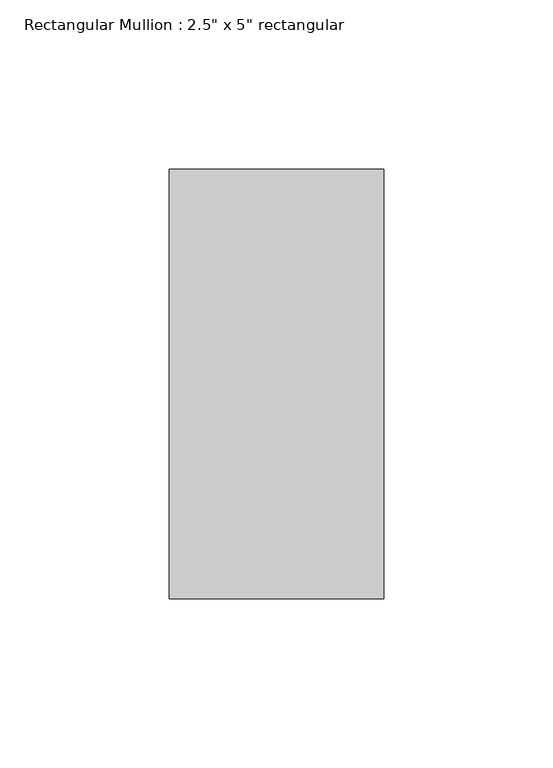
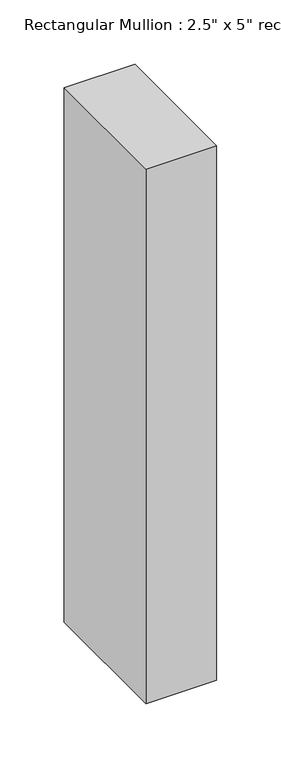
"""IFC4 building model written with IfcOpenShell, lengths in millimetres: member geometry."""

from ifc_helpers import new_model, si_unit, frame, origin, place, context, project, spatial, polyline, outline, extrude, source, transform, mapped, element, save


def member_de31af64(model_context):
    return source(origin(), model_context, "Body", "SweptSolid", [
        extrude(outline(polyline([(0.0, 63.5), (0.0, -63.5), (-63.5, -63.5), (-63.5, 63.5), (0.0, 63.5)])), frame((0.0, 0.0, -506.9149218), z_axis=(0.0, 0.0, 1.0), x_axis=(1.0, 0.0, 0.0)), (0.0, 0.0, 1.0), 506.9149218),
    ])


if __name__ == "__main__":
    model = new_model("IFC4")
    model_context = context("Model", 3, world=origin())
    ifc_project = project(units=[si_unit("LENGTHUNIT", "METRE", prefix="MILLI")], contexts=[model_context])
    site = spatial("IfcSite", under=ifc_project)
    building = spatial("IfcBuilding", under=site)
    placement = place(None, origin())
    member_shape = member_de31af64(model_context)
    element("IfcMember", 1, ObjectType="Rectangular Mullion : 2.5\" x 5\" rectangular", at=placement, inside=building, context=model_context, shape_type="MappedRepresentation", body=[
        mapped(member_shape, transform((0.0, 0.0, 0.0), x_axis=(1.0, 0.0, 0.0), y_axis=(0.0, 1.0, 0.0), z_axis=(0.0, 0.0, 1.0))),
    ])
    save(model, "model.ifc")

# Revit data of these elements
# Type "Rectangular Mullion : 2.5\" x 5\" rectangular"
#   built-in parameter 1007304 = 0.416667 (stored number, unit not read)
#   built-in parameter 1007301 = 0.104167 (stored number, unit not read)
#   built-in parameter 1007300 = 0.104167 (stored number, unit not read)
